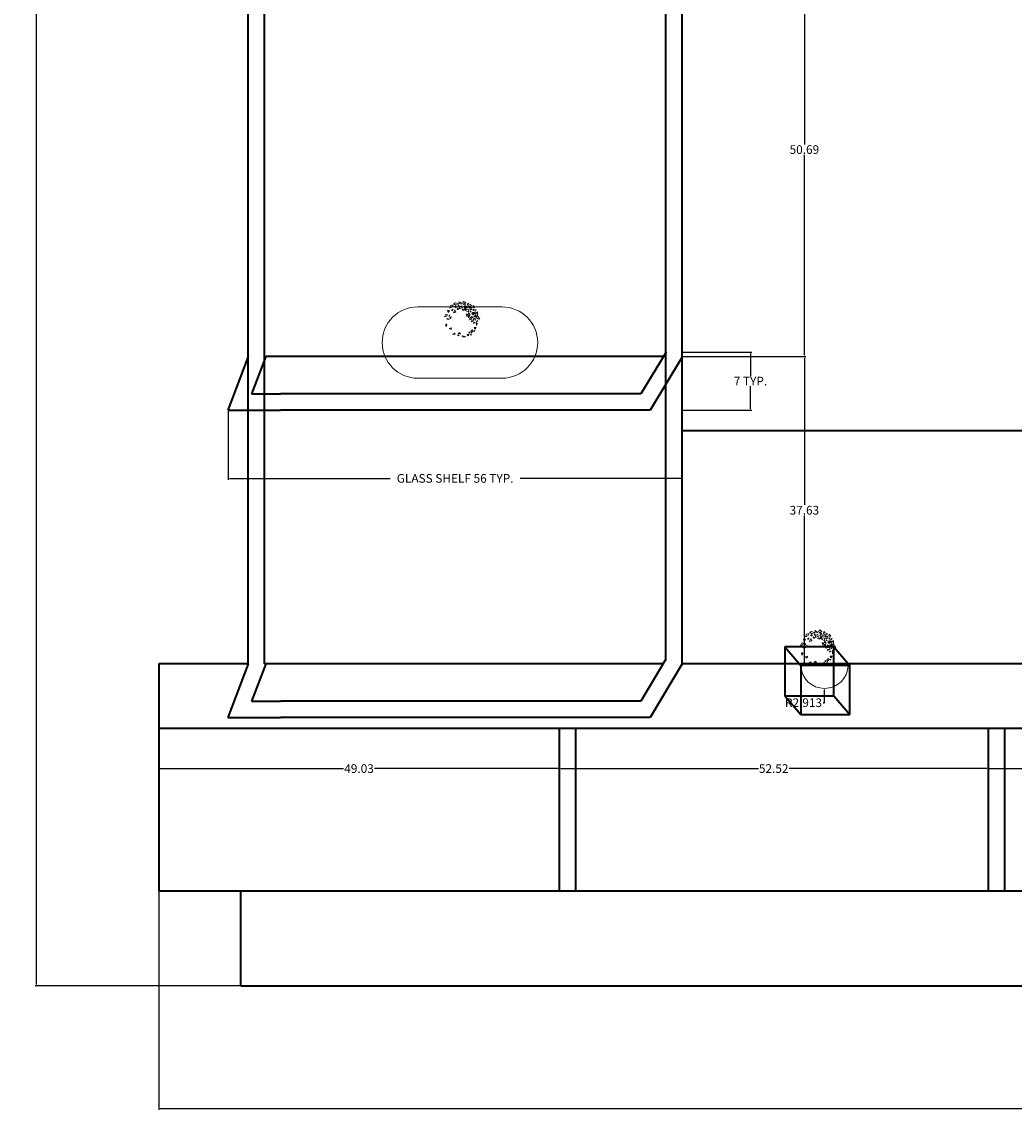
# Model space of a CAD drawing. Units: inches. Extents: x 35 to 365, y 67 to 380.
# Tile 1 of 5: x 35 to 156, y 67 to 201. Entities that reach past the tile are written whole.
import ezdxf

# ---------------------------------------------------------------- set-up
doc = ezdxf.new("R2010")
doc.units = ezdxf.units.IN
doc.header["$MEASUREMENT"] = 0
for name, color, linetype, lineweight in [('A-ANNO-DIMS', 2, 'Continuous', 18), ('A-FURN', 7, 'Continuous', 35), ('A-FURN-PLNT', 3, 'Continuous', 13)]:
    doc.layers.add(name, color=color, linetype=linetype, lineweight=lineweight)
doc.styles.get("Standard").update_dxf_attribs({"font": 'arial.ttf'})
doc.dimstyles.get("Standard").update_dxf_attribs({"dimtxt": 1.0625, "dimasz": 0.18, "dimexe": 0.18, "dimexo": 0.0625, "dimgap": 0.09, "dimtad": 0, "dimtih": 1, "dimtoh": 1, "dimdec": 4, "dimzin": 0, "dimdsep": 46, "dimlunit": 4, "dimtxsty": 'Standard', "dimcen": 0.09, "dimadec": 0, "dimazin": 0, "dimtfac": 1, "dimtdec": 4, "dimtofl": 0, "dimtmove": 0, "dimatfit": 3, "dimfxl": 1, "dimtolj": 1, "dimtzin": 0, "dimarcsym": 0})

# ---------------------------------------------------------------- blocks, each defined once
blk = doc.blocks.new('*U2')
for points in [[(-5.78, 9.75), (-7.54, 9.23), (-8.01, 7.5), (-6.26, 8.45)], [(-4.43, 11.05), (-5.18, 10.36), (-3.96, 9.49), (-2.07, 10.36)], [(-4.84, 8.63), (-3.83, 7.85), (-4.03, 8.97)], [(-2.88, 7.5), (-3.15, 6.64), (-2.27, 6.72)], [(-1.94, 9.49), (-2.48, 8.97), (-2.27, 8.54), (-1.8, 9.06)], [(-2, 11.66), (-1.6, 10.62), (-0.52, 10.1), (-0.18, 10.62), (-0.79, 10.96)], [(0.02, 9.06), (-1.33, 8.54), (-1.73, 7.16), (0.29, 7.76)], [(1.24, 12), (0.56, 11.31), (0.76, 10.01), (2.52, 11.05)], [(1.37, 8.54), (3.13, 8.8), (3.8, 7.85), (1.91, 7.76)], [(2.59, 9.93), (1.84, 9.75), (1.64, 9.23), (2.32, 9.41)], [(1.71, 6.29), (1.71, 7.07), (2.65, 7.5), (2.11, 6.9)], [(4.14, 11.14), (3.6, 10.01), (4, 9.23), (5.22, 8.71), (6.3, 9.41), (5.08, 10.19), (4.61, 10.01)], [(4.61, 8.28), (4.54, 7.76), (4.95, 7.59), (4.95, 8.28)], [(6.43, 7.94), (5.49, 7.68), (5.56, 6.21), (6.5, 6.64)], [(7.45, 9.32), (7.11, 7.94), (8.52, 7.94)], [(-11.32, 1.79), (-9.83, 2.31), (-9.63, 3.44), (-10.44, 3.52)], [(-8.21, 0.41), (-9.43, 0.32), (-9.83, 0.84)], [(-8.14, 6.03), (-9.36, 5.95), (-9.02, 4.73)], [(-8.21, 3.09), (-8.48, 2.31), (-7.87, 2.57)], [(-7, 1.79), (-7.94, 1.53), (-7.47, 0.49)], [(-5.78, 6.81), (-6.66, 6.21), (-6.52, 5.69)], [(-4.57, 6.38), (-5.45, 4.47), (-3.89, 4.82)], [(0.76, 7.16), (0.09, 6.46), (1.1, 5.95)], [(2.52, 6.81), (2.52, 5.86), (4.41, 5.17), (4.61, 6.72)], [(3.53, 1.88), (2.86, 3.52), (3.8, 3.52)], [(4.41, 4.56), (4.27, 3.7), (5.49, 3.26)], [(4.27, 2.74), (5.29, 2.66), (4.41, 1.27)], [(5.83, 1.53), (5.02, 0.41), (5.49, -0.02), (6.5, 0.41)], [(5.49, 5.51), (5.42, 4.82), (6.16, 5.08)], [(7.51, 1.71), (6.91, 1.27), (6.23, 2.14)], [(8.12, 4.99), (7.11, 4.65), (6.5, 4.13), (7.38, 3.09), (8.12, 3.52), (7.65, 3.87)], [(7.85, 6.81), (7.18, 6.21), (9, 5.51), (9.33, 6.38)], [(8.12, 0.75), (7.51, 0.15), (8.93, -0.28), (9.13, 0.49)], [(8.19, 2.57), (7.92, 2.05), (8.66, 1.53)], [(8.73, 4.73), (8.19, 4.56), (8.39, 3.87), (8.59, 4.04)], [(10.28, 5.17), (9.2, 4.04), (9, 2.31), (10.48, 0.49), (11.76, 0.41), (10.35, 2.48), (9.33, 2.4), (10.28, 2.83)], [(-10.03, -2.71), (-10.64, -3.31), (-10.44, -4.44), (-9.9, -3.49)], [(-8.28, -5.73), (-6.79, -5.3), (-7, -6.51)], [(6.1, -8.94), (6.16, -7.21), (6.91, -6.69), (7.24, -7.38)], [(7.78, -0.8), (6.43, -1.5), (6.43, -0.72)], [(8.32, -1.75), (7.98, -2.53), (7.58, -2.1)], [(8.05, -8.07), (8.59, -7.12), (7.92, -7.55)], [(9.33, -5.13), (8.46, -6.25), (7.98, -5.22)], [(9.33, -1.75), (9.54, -3.74), (10.14, -2.53)], [(10.08, -0.63), (9.74, -1.32), (10.48, -0.89)], [(-4.84, -8.85), (-4.43, -9.45), (-5.99, -9.8)], [(-2.54, -10.06), (-3.02, -10.23), (-1.8, -10.67)], [(-2.34, -9.2), (-1.26, -8.5), (-0.99, -9.54)], [(0.22, -10.58), (0.83, -11.27), (2.59, -11.36)], [(4.07, -9.45), (3.53, -9.97), (4.07, -10.58), (4.61, -9.89)], [(5.29, -7.98), (4.61, -8.16), (5.02, -8.94)], [(6.03, -9.45), (5.42, -9.97), (6.16, -10.15)]]:
    blk.add_lwpolyline(points, close=True)
blk = doc.blocks.new('SHELF-GLASS')
for p, q in [((53.63, 7.13), (50.54, 2)), ((2.48, 6.58), (0, 0)), ((4.62, 6.58), (2.89, 2)), ((53.29, 6.58), (4.62, 6.58)), ((55.63, 6.58), (51.68, 0)), ((2.89, 2), (6.44, 2)), ((50.54, 2), (6.44, 2)), ((0, 0), (6.44, 0)), ((51.68, 0), (6.44, 0))]:
    blk.add_line(p, q)
blk = doc.blocks.new('PLANTER')
for points in [[(4.37, 8.73), (14.67, 8.73)], [(14.67, 0), (4.37, 0)]]:
    blk.add_lwpolyline(points)
for centre, start, end in [((4.37, 4.37), 90, 270), ((14.67, 4.37), 270, 90)]:
    blk.add_arc(centre, 4.37, start, end)
blk = doc.blocks.new('*D7')
at = {"layer": 'A-ANNO-DIMS', "color": 0, "lineweight": -2, "transparency": 16777216}
for p, q in [((59.76, 153.47), (59.76, 145.01)), ((115.38, 153.47), (115.38, 145.01)), ((59.94, 145.19), (79.62, 145.19)), ((115.2, 145.19), (95.52, 145.19))]:
    blk.add_line(p, q, dxfattribs=at)
at = {"layer": 'A-ANNO-DIMS', "color": 0, "transparency": 16777216}
for points in [[(59.94, 145.22), (59.94, 145.16), (59.76, 145.19)], [(115.2, 145.22), (115.2, 145.16), (115.38, 145.19)]]:
    blk.add_solid(points, dxfattribs=at)
at = {"layer": 'Defpoints', "color": 0, "transparency": 16777216}
for p in [(59.76, 153.53), (115.38, 153.53), (115.38, 145.19)]:
    blk.add_point(p, dxfattribs=at)
at = {"layer": 'A-ANNO-DIMS', "color": 0, "transparency": 16777216, "insert": (87.57, 145.19), "char_height": 1.0625, "attachment_point": 5}
blk.add_mtext('\\A1;GLASS SHELF 56 TYP.', dxfattribs=at)
blk = doc.blocks.new('*D8')
at = {"layer": 'A-ANNO-DIMS', "color": 0, "lineweight": -2, "transparency": 16777216}
for p, q in [((115.45, 160.66), (123.91, 160.66)), ((123.73, 160.48), (123.73, 157.72)), ((123.73, 153.71), (123.73, 156.48)), ((115.45, 153.53), (123.91, 153.53))]:
    blk.add_line(p, q, dxfattribs=at)
at = {"layer": 'A-ANNO-DIMS', "color": 0, "transparency": 16777216}
for points in [[(123.7, 160.48), (123.76, 160.48), (123.73, 160.66)], [(123.7, 153.71), (123.76, 153.71), (123.73, 153.53)]]:
    blk.add_solid(points, dxfattribs=at)
at = {"layer": 'Defpoints', "color": 0, "transparency": 16777216}
for p in [(115.38, 160.66), (123.73, 160.66), (115.38, 153.53)]:
    blk.add_point(p, dxfattribs=at)
at = {"layer": 'A-ANNO-DIMS', "color": 0, "transparency": 16777216, "insert": (123.73, 157.1), "char_height": 1.062, "attachment_point": 5}
blk.add_mtext('\\A1;7 TYP.', dxfattribs=at)
blk = doc.blocks.new('*D9')
at = {"layer": 'A-ANNO-DIMS', "color": 0, "lineweight": -2, "transparency": 16777216}
for p, q in [((51.28, 94.63), (51.28, 67.85)), ((347.67, 82.99), (347.67, 67.85)), ((51.46, 68.03), (197.58, 68.03)), ((347.49, 68.03), (201.36, 68.03))]:
    blk.add_line(p, q, dxfattribs=at)
at = {"layer": 'A-ANNO-DIMS', "color": 0, "transparency": 16777216}
for points in [[(51.46, 68.06), (51.46, 68), (51.28, 68.03)], [(347.49, 68.06), (347.49, 68), (347.67, 68.03)]]:
    blk.add_solid(points, dxfattribs=at)
at = {"layer": 'Defpoints', "color": 0, "transparency": 16777216}
for p in [(51.28, 94.7), (347.67, 83.05), (347.67, 68.03)]:
    blk.add_point(p, dxfattribs=at)
at = {"layer": 'A-ANNO-DIMS', "color": 0, "transparency": 16777216, "insert": (199.47, 68.03), "char_height": 1.062, "attachment_point": 5}
blk.add_mtext('\\A1;296.4', dxfattribs=at)
blk = doc.blocks.new('*D10')
at = {"layer": 'A-ANNO-DIMS', "color": 0, "lineweight": -2, "transparency": 16777216}
for p, q in [((61.75, 351.36), (36.15, 351.36)), ((36.33, 351.18), (36.33, 217.84)), ((36.33, 83.23), (36.33, 216.57)), ((61.26, 83.05), (36.15, 83.05))]:
    blk.add_line(p, q, dxfattribs=at)
at = {"layer": 'A-ANNO-DIMS', "color": 0, "transparency": 16777216}
for points in [[(36.3, 351.18), (36.36, 351.18), (36.33, 351.36)], [(36.3, 83.23), (36.36, 83.23), (36.33, 83.05)]]:
    blk.add_solid(points, dxfattribs=at)
at = {"layer": 'Defpoints', "color": 0, "transparency": 16777216}
for p in [(36.33, 351.36), (61.82, 351.36), (61.32, 83.05)]:
    blk.add_point(p, dxfattribs=at)
at = {"layer": 'A-ANNO-DIMS', "color": 0, "transparency": 16777216, "insert": (36.33, 217.21), "char_height": 1.062, "attachment_point": 5}
blk.add_mtext('\\A1;268.3', dxfattribs=at)
blk = doc.blocks.new('*D16')
at = {"layer": 'A-ANNO-DIMS', "color": 0, "lineweight": -2, "transparency": 16777216}
for p, q in [((51.28, 94.76), (51.28, 109.83)), ((100.31, 94.76), (100.31, 109.83)), ((51.46, 109.65), (73.89, 109.65)), ((100.13, 109.65), (77.7, 109.65))]:
    blk.add_line(p, q, dxfattribs=at)
at = {"layer": 'A-ANNO-DIMS', "color": 0, "transparency": 16777216}
for points in [[(51.46, 109.68), (51.46, 109.62), (51.28, 109.65)], [(100.13, 109.68), (100.13, 109.62), (100.31, 109.65)]]:
    blk.add_solid(points, dxfattribs=at)
at = {"layer": 'Defpoints', "color": 0, "transparency": 16777216}
for p in [(100.31, 109.65), (51.28, 94.7), (100.31, 94.7)]:
    blk.add_point(p, dxfattribs=at)
at = {"layer": 'A-ANNO-DIMS', "color": 0, "transparency": 16777216, "insert": (75.8, 109.65), "char_height": 1.062, "attachment_point": 5}
blk.add_mtext('\\A1;49.03', dxfattribs=at)
blk = doc.blocks.new('*D17')
at = {"layer": 'A-ANNO-DIMS', "color": 0, "lineweight": -2, "transparency": 16777216}
for p, q in [((100.31, 94.76), (100.31, 109.83)), ((152.83, 94.76), (152.83, 109.83)), ((100.49, 109.65), (124.7, 109.65)), ((152.65, 109.65), (128.45, 109.65))]:
    blk.add_line(p, q, dxfattribs=at)
at = {"layer": 'A-ANNO-DIMS', "color": 0, "transparency": 16777216}
for points in [[(100.49, 109.68), (100.49, 109.62), (100.31, 109.65)], [(152.65, 109.68), (152.65, 109.62), (152.83, 109.65)]]:
    blk.add_solid(points, dxfattribs=at)
at = {"layer": 'Defpoints', "color": 0, "transparency": 16777216}
for p in [(152.83, 109.65), (100.31, 94.7), (152.83, 94.7)]:
    blk.add_point(p, dxfattribs=at)
at = {"layer": 'A-ANNO-DIMS', "color": 0, "transparency": 16777216, "insert": (126.57, 109.65), "char_height": 1.062, "attachment_point": 5}
blk.add_mtext('\\A1;52.52', dxfattribs=at)
blk = doc.blocks.new('*D18')
at = {"layer": 'A-ANNO-DIMS', "color": 0, "lineweight": -2, "transparency": 16777216}
for p, q in [((152.83, 94.76), (152.83, 109.83)), ((209.69, 94.76), (209.69, 109.83)), ((153.01, 109.65), (179.38, 109.65)), ((209.51, 109.65), (183.14, 109.65))]:
    blk.add_line(p, q, dxfattribs=at)
at = {"layer": 'A-ANNO-DIMS', "color": 0, "transparency": 16777216}
for points in [[(153.01, 109.68), (153.01, 109.62), (152.83, 109.65)], [(209.51, 109.68), (209.51, 109.62), (209.69, 109.65)]]:
    blk.add_solid(points, dxfattribs=at)
at = {"layer": 'Defpoints', "color": 0, "transparency": 16777216}
for p in [(209.69, 109.65), (152.83, 94.7), (209.69, 94.7)]:
    blk.add_point(p, dxfattribs=at)
at = {"layer": 'A-ANNO-DIMS', "color": 0, "transparency": 16777216, "insert": (181.26, 109.65), "char_height": 1.062, "attachment_point": 5}
blk.add_mtext('\\A1;56.86', dxfattribs=at)
blk = doc.blocks.new('*D34')
at = {"layer": 'A-ANNO-DIMS', "color": 0, "lineweight": -2, "transparency": 16777216}
for p, q in [((115.45, 160.11), (130.51, 160.11)), ((130.33, 159.93), (130.33, 141.93)), ((130.33, 122.66), (130.33, 140.66)), ((115.45, 122.48), (130.51, 122.48))]:
    blk.add_line(p, q, dxfattribs=at)
at = {"layer": 'A-ANNO-DIMS', "color": 0, "transparency": 16777216}
for points in [[(130.3, 159.93), (130.36, 159.93), (130.33, 160.11)], [(130.3, 122.66), (130.36, 122.66), (130.33, 122.48)]]:
    blk.add_solid(points, dxfattribs=at)
at = {"layer": 'Defpoints', "color": 0, "transparency": 16777216}
for p in [(115.38, 160.11), (115.38, 122.48), (130.33, 122.48)]:
    blk.add_point(p, dxfattribs=at)
at = {"layer": 'A-ANNO-DIMS', "color": 0, "transparency": 16777216, "insert": (130.33, 141.29), "char_height": 1.062, "attachment_point": 5}
blk.add_mtext('\\A1;37.63', dxfattribs=at)
blk = doc.blocks.new('*D35')
at = {"layer": 'A-ANNO-DIMS', "color": 0, "lineweight": -2, "transparency": 16777216}
for p, q in [((115.45, 210.8), (130.51, 210.8)), ((130.33, 210.62), (130.33, 186.09)), ((130.33, 160.29), (130.33, 184.82)), ((115.45, 160.11), (130.51, 160.11))]:
    blk.add_line(p, q, dxfattribs=at)
at = {"layer": 'A-ANNO-DIMS', "color": 0, "transparency": 16777216}
for points in [[(130.3, 210.62), (130.36, 210.62), (130.33, 210.8)], [(130.3, 160.29), (130.36, 160.29), (130.33, 160.11)]]:
    blk.add_solid(points, dxfattribs=at)
at = {"layer": 'Defpoints', "color": 0, "transparency": 16777216}
for p in [(115.38, 210.8), (115.38, 160.11), (130.33, 160.11)]:
    blk.add_point(p, dxfattribs=at)
at = {"layer": 'A-ANNO-DIMS', "color": 0, "transparency": 16777216, "insert": (130.33, 185.46), "char_height": 1.062, "attachment_point": 5}
blk.add_mtext('\\A1;50.69', dxfattribs=at)
blk = doc.blocks.new('*D39')
at = {"layer": 'A-ANNO-DIMS', "color": 0, "lineweight": -2, "transparency": 16777216}
for p, q in [((132.7, 122.38), (132.88, 122.38)), ((132.79, 122.29), (132.79, 122.47)), ((132.79, 117.72), (132.79, 119.28)), ((132.61, 117.72), (132.79, 117.72))]:
    blk.add_line(p, q, dxfattribs=at)
at = {"layer": 'A-ANNO-DIMS', "color": 0, "transparency": 16777216}
blk.add_solid([(132.76, 119.28), (132.82, 119.28), (132.79, 119.46)], dxfattribs=at)
at = {"layer": 'Defpoints', "color": 0, "transparency": 16777216}
for p in [(132.79, 122.38), (132.79, 119.46)]:
    blk.add_point(p, dxfattribs=at)
at = {"layer": 'A-ANNO-DIMS', "color": 0, "transparency": 16777216, "insert": (130.22, 117.72), "char_height": 1.062, "attachment_point": 5}
blk.add_mtext('\\A1;R2.913', dxfattribs=at)

msp = doc.modelspace()

# ---------------------------------------------------------------- linework, layer by layer
at = {"layer": 'A-FURN'}
for p, q in [((62.2395, 122.4805), (62.2395, 350.3365)), ((64.2395, 122.4805), (64.2395, 350.3365)), ((113.383, 123.0351), (113.383, 350.3365)), ((115.383, 122.4805), (115.383, 350.3365)), ((127.9355, 124.5549), (127.9355, 118.5549)), ((133.9355, 124.5549), (127.9355, 124.5549)), ((127.9355, 124.5549), (129.8823, 122.2723)), ((133.9355, 118.5549), (133.9355, 124.5549)), ((133.9355, 124.5549), (135.8823, 122.2723)), ((51.2797, 122.4805), (51.2797, 114.5646)), ((62.2395, 122.4805), (51.2797, 122.4805)), ((62.2395, 122.4805), (59.756, 115.903)), ((64.3773, 122.4805), (62.649, 117.903)), ((113.0498, 122.4805), (64.2395, 122.4805)), ((113.383, 123.0351), (110.2998, 117.903)), ((115.383, 122.4805), (111.4314, 115.903)), ((323.6655, 122.4805), (115.383, 122.4805)), ((129.8823, 122.2723), (129.8823, 116.2723)), ((135.8823, 122.2723), (129.8823, 122.2723)), ((135.8823, 116.2723), (135.8823, 122.2723)), ((62.649, 117.903), (66.1912, 117.903)), ((110.2998, 117.903), (66.1912, 117.903)), ((127.9355, 118.5549), (133.9355, 118.5549)), ((127.9355, 118.5549), (129.8823, 116.2723)), ((133.9355, 118.5549), (135.8823, 116.2723)), ((59.756, 115.903), (66.1912, 115.903)), ((111.4314, 115.903), (66.1912, 115.903)), ((129.8823, 116.2723), (135.8823, 116.2723)), ((323.6655, 114.5646), (51.2797, 114.5646)), ((51.2797, 114.5646), (51.2797, 94.6954)), ((100.3126, 114.5646), (100.3126, 94.6954)), ((102.3126, 114.5646), (102.3126, 94.6954)), ((152.8319, 114.5646), (152.8319, 94.6954)), ((154.8319, 114.5646), (154.8319, 94.6954)), ((51.2797, 94.6954), (323.6655, 94.6954)), ((61.3227, 83.0529), (61.3227, 94.6954)), ((61.3227, 83.0529), (347.6655, 83.0529))]:
    msp.add_line(p, q, dxfattribs=at)
msp.add_lwpolyline([(115.383, 254.0695), (323.6655, 254.0695), (323.6655, 151.0198), (115.383, 151.0198)], close=True, dxfattribs=at)
at = {"layer": 'A-FURN-PLNT'}
msp.add_arc((132.7935, 122.3764), 2.9131, 182.048203, 357.951797, dxfattribs=at)

# ---------------------------------------------------------------- block references
at = {"layer": 'A-FURN'}
msp.add_blockref('SHELF-GLASS', (59.756, 153.531), dxfattribs=at)
at = {"layer": 'A-FURN-PLNT', "rotation": 180}
msp.add_blockref('PLANTER', (97.6775, 166.1941), dxfattribs=at)
at = {"layer": 'A-FURN-PLNT', "xscale": 0.1863493069736422, "yscale": 0.1863493069736422, "zscale": 0.1863493069736422}
for p in [(88.3937, 164.629), (131.978, 124.386)]:
    msp.add_blockref('*U2', p, dxfattribs=at)

# ---------------------------------------------------------------- dimensions: what is measured, and where the dimension line sits
at = {"layer": 'A-ANNO-DIMS'}
for base, p1, p2, angle, override, picture, middle in [((36.3297, 351.3604), (61.3227, 83.0529), (61.8154, 351.3604), 90, {"dimdec": 1, "dimlfac": 1, "dimrnd": 0, "dimzin": 0, "dimdsep": 46, "dimlunit": 2}, '*D10', (36.3297, 217.2067)), ((130.333, 160.1089), (115.383, 210.8028), (115.383, 160.1089), 270, {"dimdec": 2, "dimlfac": 1, "dimrnd": 0, "dimzin": 0, "dimdsep": 46, "dimlunit": 2}, '*D35', (130.333, 185.4559)), ((130.333, 122.4805), (115.383, 160.1089), (115.383, 122.4805), 270, {"dimdec": 2, "dimlfac": 1, "dimrnd": 0, "dimzin": 0, "dimdsep": 46, "dimlunit": 2}, '*D34', (130.333, 141.2947)), ((209.6918, 109.6454), (152.8319, 94.6954), (209.6918, 94.6954), 0, {"dimdec": 2, "dimlfac": 1, "dimrnd": 0, "dimzin": 0, "dimdsep": 46, "dimlunit": 2}, '*D18', (181.2619, 109.6454))]:
    dim = msp.add_linear_dim(base=base, p1=p1, p2=p2, angle=angle, dimstyle='Standard', override=override, dxfattribs=at)
    dim.commit()
    dim.dimension.update_dxf_attribs({"geometry": picture, "text_midpoint": middle})
dim = msp.add_linear_dim(base=(123.7271, 160.6635), p1=(115.383, 153.5314), p2=(115.383, 160.6635), angle=90, text='<> TYP.', dimstyle='Standard', override={"dimdec": 0, "dimrnd": 0, "dimzin": 0, "dimlunit": 2}, dxfattribs=at)
dim.commit()
dim.dimension.update_dxf_attribs({"geometry": '*D8', "text_midpoint": (123.7271, 157.0974)})
dim = msp.add_linear_dim(base=(115.383, 145.1873), p1=(59.756, 153.5314), p2=(115.383, 153.5314), text='GLASS SHELF <> TYP.', dimstyle='Standard', override={"dimdec": 0, "dimrnd": 0, "dimzin": 0, "dimlunit": 2}, dxfattribs=at)
dim.commit()
dim.dimension.update_dxf_attribs({"geometry": '*D7', "text_midpoint": (87.5695, 145.1873)})
dim = msp.add_radius_dim(center=(132.7935, 122.3764), mpoint=(132.793, 119.4634), dimstyle='Standard', override={"dimdec": 3, "dimlfac": 1, "dimrnd": 0, "dimzin": 0, "dimdsep": 46, "dimlunit": 2}, dxfattribs=at)
dim.commit()
dim.dimension.update_dxf_attribs({"geometry": '*D39', "text_midpoint": (130.2216, 117.7155), "dimtype": 164})
for base, p1, p2, override, picture, middle in [((100.3126, 109.6454), (51.2797, 94.6954), (100.3126, 94.6954), {"dimdec": 2, "dimlfac": 1, "dimrnd": 0, "dimzin": 0, "dimdsep": 46, "dimlunit": 2}, '*D16', (75.7961, 109.6454)), ((152.8319, 109.6454), (100.3126, 94.6954), (152.8319, 94.6954), {"dimdec": 2, "dimlfac": 1, "dimrnd": 0, "dimzin": 0, "dimdsep": 46, "dimlunit": 2}, '*D17', (126.5723, 109.6454)), ((347.6655, 68.0268), (51.2797, 94.6954), (347.6655, 83.0529), {"dimdec": 1, "dimlfac": 1, "dimrnd": 0, "dimzin": 0, "dimdsep": 46, "dimlunit": 2}, '*D9', (199.4726, 68.0268))]:
    dim = msp.add_linear_dim(base=base, p1=p1, p2=p2, dimstyle='Standard', override=override, dxfattribs=at)
    dim.commit()
    dim.dimension.update_dxf_attribs({"geometry": picture, "text_midpoint": middle})

doc.saveas('drawing.dxf')
